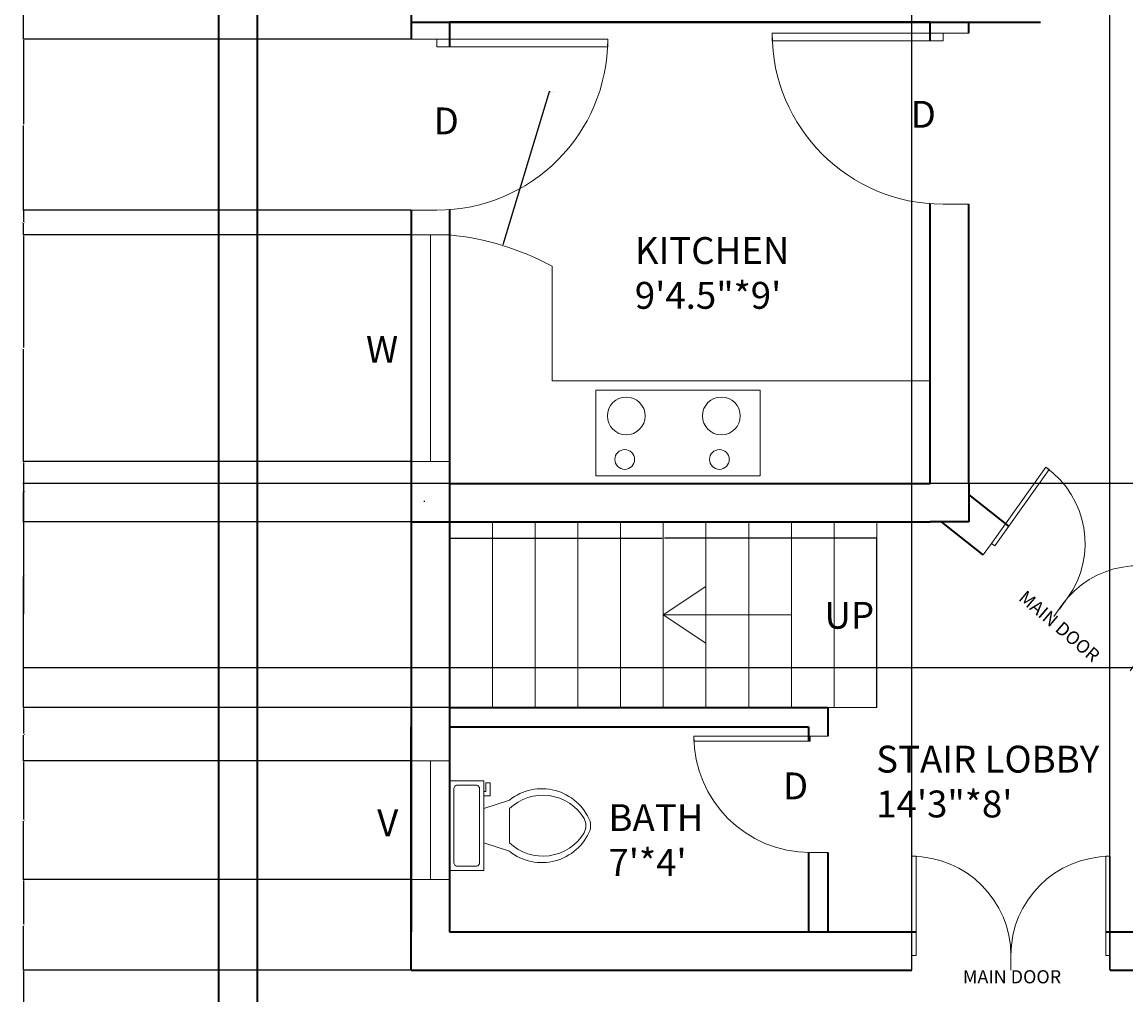
# Model space of a CAD drawing. Units: inches. Extents: x 2284 to 2815, y 1123 to 1948.
# Tile 2 of 6: x 2284 to 2543, y 1414 to 1641. Entities that reach past the tile are written whole.
import ezdxf

# ---------------------------------------------------------------- set-up
doc = ezdxf.new("R2010")
doc.units = ezdxf.units.IN
for name, color, linetype, lineweight in [('A-ANNO-DIMS', 2, 'Continuous', 18), ('A-ANNO-SYMB', 30, 'Continuous', 18), ('A-AREA-IDEN', 30, 'Continuous', 18), ('A-EQPM', 10, 'Continuous', 18), ('A-FLOR-CASE', 8, 'Continuous', 18), ('A-FLOR-FIXT', 9, 'Continuous', 18), ('A-FLOR-STRS', 7, 'Continuous', 18), ('A-WALL-PATT', 140, 'Continuous', 13), ('C-SITE-WALL', 7, 'Continuous', 35), ('DOOR', 190, 'Continuous', 18), ('TEXT', 30, 'Continuous', 18), ('WALL', 7, 'Continuous', 35), ('WIND', 210, 'Continuous', 18)]:
    doc.layers.add(name, color=color, linetype=linetype, lineweight=lineweight)
doc.styles.get("Standard").update_dxf_attribs({"font": 'arial.ttf'})
doc.dimstyles.get("Standard").update_dxf_attribs({"dimtxt": 0.18, "dimasz": 0.18, "dimexe": 0.18, "dimexo": 0.0625, "dimgap": 0.09, "dimtad": 0, "dimtih": 1, "dimtoh": 1, "dimdec": 4, "dimzin": 0, "dimdsep": 46, "dimtxsty": 'Standard', "dimcen": 0.09, "dimadec": 0, "dimazin": 0, "dimtfac": 1, "dimtdec": 4, "dimtofl": 0, "dimtmove": 0, "dimatfit": 3, "dimfxl": 1, "dimtolj": 1, "dimtzin": 0, "dimarcsym": 0})

# ---------------------------------------------------------------- blocks, each defined once
blk = doc.blocks.new('*U2')
for p, q in [((0, 0), (0, -6)), ((40, 0), (40, -6))]:
    blk.add_line(p, q)
blk.add_lwpolyline([(0, 0), (0, 40), (1.75, 40), (1.75, 0)], close=True)
blk.add_arc((0, 0), 40, 0, 90)
blk = doc.blocks.new('*U4')
for p, q in [((9.5, -6), (9.5, -2)), ((-10, -8.5), (-8, -8.5)), ((-10, -9.5), (-10, -8.5)), ((-7, -9.5), (-10, -9.5)), ((-8, -8.5), (-8, -8)), ((-7, -8), (-7, -9.5)), ((-4, -8), (-6, -14)), ((4, -8), (6, -14)), ((4, -14), (-4, -14))]:
    blk.add_line(p, q)
blk.add_lwpolyline([(10.5, -8), (10.5, 0), (-10.5, 0), (-10.5, -8)], close=True)
for points in [[(-9.5, -2), (-9.5, -6)], [(8.5, -1), (-8.5, -1)], [(-8.5, -7), (8.5, -7)]]:
    blk.add_lwpolyline(points)
for centre, radius, start, end in [((-8.62, -1.88), 0.884, 81.8699, 188.1301), ((8.62, -1.88), 0.884, 351.8699, 98.1301), ((-8.62, -6.12), 0.884, 171.8699, 278.1301), ((8.62, -6.12), 0.884, 261.8699, 8.1301), ((3.52, -21.58), 12.17, 141.4691, 247.9714), ((4.2, -21.82), 11.33, 136.3677, 238.9468), ((-3.52, -21.58), 12.17, 292.0284, 38.5307), ((-4.2, -21.82), 11.33, 301.053, 43.6321), ((0, -27.88), 4, 245.7318, 294.2682), ((0, -29), 4, 254.8605, 285.1395)]:
    blk.add_arc(centre, radius, start, end)
blk = doc.blocks.new('*D23')
at = {"layer": 'A-ANNO-DIMS', "color": 0, "lineweight": -2, "transparency": 16777216}
for p, q in [((2375.49, 1419.4), (2284.67, 1419.4)), ((2284.85, 1419.22), (2284.85, 1334.09)), ((2284.85, 1248.6), (2284.85, 1333.73)), ((2339.49, 1248.42), (2284.67, 1248.42))]:
    blk.add_line(p, q, dxfattribs=at)
at = {"layer": 'A-ANNO-DIMS', "color": 0, "transparency": 16777216}
for points in [[(2284.82, 1419.22), (2284.88, 1419.22), (2284.85, 1419.4)], [(2284.82, 1248.6), (2284.88, 1248.6), (2284.85, 1248.42)]]:
    blk.add_solid(points, dxfattribs=at)
at = {"layer": 'Defpoints', "color": 0, "transparency": 16777216}
for p in [(2284.85, 1419.4), (2375.55, 1419.4), (2339.55, 1248.42)]:
    blk.add_point(p, dxfattribs=at)
at = {"layer": 'A-ANNO-DIMS', "color": 0, "transparency": 16777216, "insert": (2284.85, 1333.91), "char_height": 0.18, "attachment_point": 5}
blk.add_mtext('\\A1;171', dxfattribs=at)
blk = doc.blocks.new('*D24')
at = {"layer": 'A-ANNO-DIMS', "color": 0, "lineweight": -2, "transparency": 16777216}
for p, q in [((2375.49, 1440.64), (2284.67, 1440.64)), ((2284.85, 1440.46), (2284.85, 1430.2)), ((2284.85, 1419.58), (2284.85, 1429.84)), ((2375.49, 1419.4), (2284.67, 1419.4))]:
    blk.add_line(p, q, dxfattribs=at)
at = {"layer": 'A-ANNO-DIMS', "color": 0, "transparency": 16777216}
for points in [[(2284.82, 1440.46), (2284.88, 1440.46), (2284.85, 1440.64)], [(2284.82, 1419.58), (2284.88, 1419.58), (2284.85, 1419.4)]]:
    blk.add_solid(points, dxfattribs=at)
at = {"layer": 'Defpoints', "color": 0, "transparency": 16777216}
for p in [(2284.85, 1440.64), (2375.55, 1440.64), (2375.55, 1419.4)]:
    blk.add_point(p, dxfattribs=at)
at = {"layer": 'A-ANNO-DIMS', "color": 0, "transparency": 16777216, "insert": (2284.85, 1430.02), "char_height": 0.18, "attachment_point": 5}
blk.add_mtext('\\A1;21.24', dxfattribs=at)
blk = doc.blocks.new('*D25')
at = {"layer": 'A-ANNO-DIMS', "color": 0, "lineweight": -2, "transparency": 16777216}
for p, q in [((2375.49, 1468.42), (2284.67, 1468.42)), ((2284.85, 1468.24), (2284.85, 1454.71)), ((2284.85, 1440.82), (2284.85, 1454.35)), ((2375.49, 1440.64), (2284.67, 1440.64))]:
    blk.add_line(p, q, dxfattribs=at)
at = {"layer": 'A-ANNO-DIMS', "color": 0, "transparency": 16777216}
for points in [[(2284.82, 1468.24), (2284.88, 1468.24), (2284.85, 1468.42)], [(2284.82, 1440.82), (2284.88, 1440.82), (2284.85, 1440.64)]]:
    blk.add_solid(points, dxfattribs=at)
at = {"layer": 'Defpoints', "color": 0, "transparency": 16777216}
for p in [(2284.85, 1468.42), (2375.55, 1468.42), (2375.55, 1440.64)]:
    blk.add_point(p, dxfattribs=at)
at = {"layer": 'A-ANNO-DIMS', "color": 0, "transparency": 16777216, "insert": (2284.85, 1454.53), "char_height": 0.18, "attachment_point": 5}
blk.add_mtext('\\A1;27.78', dxfattribs=at)
blk = doc.blocks.new('*D26')
at = {"layer": 'A-ANNO-DIMS', "color": 0, "lineweight": -2, "transparency": 16777216}
for p, q in [((2384.49, 1480.9), (2284.67, 1480.9)), ((2284.85, 1480.72), (2284.85, 1474.85)), ((2284.85, 1468.6), (2284.85, 1474.48)), ((2375.49, 1468.42), (2284.67, 1468.42))]:
    blk.add_line(p, q, dxfattribs=at)
at = {"layer": 'A-ANNO-DIMS', "color": 0, "transparency": 16777216}
for points in [[(2284.82, 1480.72), (2284.88, 1480.72), (2284.85, 1480.9)], [(2284.82, 1468.6), (2284.88, 1468.6), (2284.85, 1468.42)]]:
    blk.add_solid(points, dxfattribs=at)
at = {"layer": 'Defpoints', "color": 0, "transparency": 16777216}
for p in [(2284.85, 1480.9), (2384.55, 1480.9), (2375.55, 1468.42)]:
    blk.add_point(p, dxfattribs=at)
at = {"layer": 'A-ANNO-DIMS', "color": 0, "transparency": 16777216, "insert": (2284.85, 1474.66), "char_height": 0.18, "attachment_point": 5}
blk.add_mtext('\\A1;12.48', dxfattribs=at)
blk = doc.blocks.new('*D27')
at = {"layer": 'A-ANNO-DIMS', "color": 0, "lineweight": -2, "transparency": 16777216}
for p, q in [((2384.49, 1524.4), (2284.67, 1524.4)), ((2284.85, 1524.22), (2284.85, 1502.84)), ((2284.85, 1481.08), (2284.85, 1502.47)), ((2384.49, 1480.9), (2284.67, 1480.9))]:
    blk.add_line(p, q, dxfattribs=at)
at = {"layer": 'A-ANNO-DIMS', "color": 0, "transparency": 16777216}
for points in [[(2284.82, 1524.22), (2284.88, 1524.22), (2284.85, 1524.4)], [(2284.82, 1481.08), (2284.88, 1481.08), (2284.85, 1480.9)]]:
    blk.add_solid(points, dxfattribs=at)
at = {"layer": 'Defpoints', "color": 0, "transparency": 16777216}
for p in [(2284.85, 1524.4), (2384.55, 1524.4), (2384.55, 1480.9)]:
    blk.add_point(p, dxfattribs=at)
at = {"layer": 'A-ANNO-DIMS', "color": 0, "transparency": 16777216, "insert": (2284.85, 1502.65), "char_height": 0.18, "attachment_point": 5}
blk.add_mtext('\\A1;43.5', dxfattribs=at)
blk = doc.blocks.new('*D28')
at = {"layer": 'A-ANNO-DIMS', "color": 0, "lineweight": -2, "transparency": 16777216}
for p, q in [((2375.49, 1538.49), (2284.67, 1538.49)), ((2284.85, 1538.31), (2284.85, 1531.63)), ((2284.85, 1524.58), (2284.85, 1531.26)), ((2384.49, 1524.4), (2284.67, 1524.4))]:
    blk.add_line(p, q, dxfattribs=at)
at = {"layer": 'A-ANNO-DIMS', "color": 0, "transparency": 16777216}
for points in [[(2284.82, 1538.31), (2284.88, 1538.31), (2284.85, 1538.49)], [(2284.82, 1524.58), (2284.88, 1524.58), (2284.85, 1524.4)]]:
    blk.add_solid(points, dxfattribs=at)
at = {"layer": 'Defpoints', "color": 0, "transparency": 16777216}
for p in [(2284.85, 1538.49), (2375.55, 1538.49), (2384.55, 1524.4)]:
    blk.add_point(p, dxfattribs=at)
at = {"layer": 'A-ANNO-DIMS', "color": 0, "transparency": 16777216, "insert": (2284.85, 1531.45), "char_height": 0.18, "attachment_point": 5}
blk.add_mtext('\\A1;14.086', dxfattribs=at)
blk = doc.blocks.new('*D29')
at = {"layer": 'A-ANNO-DIMS', "color": 0, "lineweight": -2, "transparency": 16777216}
for p, q in [((2375.49, 1591.56), (2284.67, 1591.56)), ((2284.85, 1591.38), (2284.85, 1565.21)), ((2284.85, 1538.67), (2284.85, 1564.84)), ((2375.49, 1538.49), (2284.67, 1538.49))]:
    blk.add_line(p, q, dxfattribs=at)
at = {"layer": 'A-ANNO-DIMS', "color": 0, "transparency": 16777216}
for points in [[(2284.82, 1591.38), (2284.88, 1591.38), (2284.85, 1591.56)], [(2284.82, 1538.67), (2284.88, 1538.67), (2284.85, 1538.49)]]:
    blk.add_solid(points, dxfattribs=at)
at = {"layer": 'Defpoints', "color": 0, "transparency": 16777216}
for p in [(2284.85, 1591.56), (2375.55, 1591.56), (2375.55, 1538.49)]:
    blk.add_point(p, dxfattribs=at)
at = {"layer": 'A-ANNO-DIMS', "color": 0, "transparency": 16777216, "insert": (2284.85, 1565.03), "char_height": 0.18, "attachment_point": 5}
blk.add_mtext('\\A1;53.07', dxfattribs=at)
blk = doc.blocks.new('*D30')
at = {"layer": 'A-ANNO-DIMS', "color": 0, "lineweight": -2, "transparency": 16777216}
for p, q in [((2375.49, 1597.37), (2284.67, 1597.37)), ((2284.85, 1597.19), (2284.85, 1594.65)), ((2284.85, 1591.74), (2284.85, 1594.29)), ((2375.49, 1591.56), (2284.67, 1591.56))]:
    blk.add_line(p, q, dxfattribs=at)
at = {"layer": 'A-ANNO-DIMS', "color": 0, "transparency": 16777216}
for points in [[(2284.82, 1597.19), (2284.88, 1597.19), (2284.85, 1597.37)], [(2284.82, 1591.74), (2284.88, 1591.74), (2284.85, 1591.56)]]:
    blk.add_solid(points, dxfattribs=at)
at = {"layer": 'Defpoints', "color": 0, "transparency": 16777216}
for p in [(2284.85, 1597.37), (2375.55, 1597.37), (2375.55, 1591.56)]:
    blk.add_point(p, dxfattribs=at)
at = {"layer": 'A-ANNO-DIMS', "color": 0, "transparency": 16777216, "insert": (2284.85, 1594.47), "char_height": 0.18, "attachment_point": 5}
blk.add_mtext('\\A1;5.807', dxfattribs=at)
blk = doc.blocks.new('*D31')
at = {"layer": 'A-ANNO-DIMS', "color": 0, "lineweight": -2, "transparency": 16777216}
for p, q in [((2375.49, 1637.37), (2284.67, 1637.37)), ((2284.85, 1637.19), (2284.85, 1617.55)), ((2284.85, 1597.55), (2284.85, 1617.19)), ((2375.49, 1597.37), (2284.67, 1597.37))]:
    blk.add_line(p, q, dxfattribs=at)
at = {"layer": 'A-ANNO-DIMS', "color": 0, "transparency": 16777216}
for points in [[(2284.82, 1637.19), (2284.88, 1637.19), (2284.85, 1637.37)], [(2284.82, 1597.55), (2284.88, 1597.55), (2284.85, 1597.37)]]:
    blk.add_solid(points, dxfattribs=at)
at = {"layer": 'Defpoints', "color": 0, "transparency": 16777216}
for p in [(2284.85, 1637.37), (2375.55, 1637.37), (2375.55, 1597.37)]:
    blk.add_point(p, dxfattribs=at)
at = {"layer": 'A-ANNO-DIMS', "color": 0, "transparency": 16777216, "insert": (2284.85, 1617.37), "char_height": 0.18, "attachment_point": 5}
blk.add_mtext('\\A1;40', dxfattribs=at)
blk = doc.blocks.new('*D32')
at = {"layer": 'A-ANNO-DIMS', "color": 0, "lineweight": -2, "transparency": 16777216}
for p, q in [((2375.49, 1678.06), (2284.67, 1678.06)), ((2284.85, 1677.88), (2284.85, 1657.9)), ((2284.85, 1637.55), (2284.85, 1657.53)), ((2375.49, 1637.37), (2284.67, 1637.37))]:
    blk.add_line(p, q, dxfattribs=at)
at = {"layer": 'A-ANNO-DIMS', "color": 0, "transparency": 16777216}
for points in [[(2284.82, 1677.88), (2284.88, 1677.88), (2284.85, 1678.06)], [(2284.82, 1637.55), (2284.88, 1637.55), (2284.85, 1637.37)]]:
    blk.add_solid(points, dxfattribs=at)
at = {"layer": 'Defpoints', "color": 0, "transparency": 16777216}
for p in [(2284.85, 1678.06), (2375.55, 1678.06), (2375.55, 1637.37)]:
    blk.add_point(p, dxfattribs=at)
at = {"layer": 'A-ANNO-DIMS', "color": 0, "transparency": 16777216, "insert": (2284.85, 1657.71), "char_height": 0.18, "attachment_point": 5}
blk.add_mtext('\\A1;40.69', dxfattribs=at)
blk = doc.blocks.new('*D46')
at = {"layer": 'A-ANNO-DIMS', "color": 0, "lineweight": -2, "transparency": 16777216}
for p, q in [((2492.72, 1419.47), (2492.72, 1948.28)), ((2539.13, 1419.47), (2539.13, 1948.28)), ((2492.9, 1948.1), (2515.54, 1948.1)), ((2538.95, 1948.1), (2516.3, 1948.1))]:
    blk.add_line(p, q, dxfattribs=at)
at = {"layer": 'A-ANNO-DIMS', "color": 0, "transparency": 16777216}
for points in [[(2492.9, 1948.13), (2492.9, 1948.07), (2492.72, 1948.1)], [(2538.95, 1948.13), (2538.95, 1948.07), (2539.13, 1948.1)]]:
    blk.add_solid(points, dxfattribs=at)
at = {"layer": 'Defpoints', "color": 0, "transparency": 16777216}
for p in [(2539.13, 1948.1), (2492.72, 1419.4), (2539.13, 1419.4)]:
    blk.add_point(p, dxfattribs=at)
at = {"layer": 'A-ANNO-DIMS', "color": 0, "transparency": 16777216, "insert": (2515.92, 1948.1), "char_height": 0.18, "attachment_point": 5}
blk.add_mtext('\\A1;46.41', dxfattribs=at)
blk = doc.blocks.new('*D55')
at = {"layer": 'A-ANNO-DIMS', "color": 0, "lineweight": -2, "transparency": 16777216}
for p, q in [((2599.47, 1533.4), (2284.67, 1533.4)), ((2284.85, 1533.22), (2284.85, 1511.99)), ((2284.85, 1490.38), (2284.85, 1511.62)), ((2555.49, 1490.2), (2284.67, 1490.2))]:
    blk.add_line(p, q, dxfattribs=at)
at = {"layer": 'A-ANNO-DIMS', "color": 0, "transparency": 16777216}
for points in [[(2284.82, 1533.22), (2284.88, 1533.22), (2284.85, 1533.4)], [(2284.82, 1490.38), (2284.88, 1490.38), (2284.85, 1490.2)]]:
    blk.add_solid(points, dxfattribs=at)
at = {"layer": 'Defpoints', "color": 0, "transparency": 16777216}
for p in [(2284.85, 1533.4), (2599.53, 1533.4), (2555.55, 1490.2)]:
    blk.add_point(p, dxfattribs=at)
at = {"layer": 'A-ANNO-DIMS', "color": 0, "transparency": 16777216, "insert": (2284.85, 1511.8), "char_height": 0.18, "attachment_point": 5}
blk.add_mtext('\\A1;43.2', dxfattribs=at)
blk = doc.blocks.new('*D56')
at = {"layer": 'A-ANNO-DIMS', "color": 0, "lineweight": -2, "transparency": 16777216}
for p, q in [((2384.55, 1480.97), (2384.55, 1520.78)), ((2384.73, 1520.6), (2434.27, 1520.6)), ((2484.37, 1520.6), (2434.83, 1520.6)), ((2484.55, 1480.97), (2484.55, 1520.78))]:
    blk.add_line(p, q, dxfattribs=at)
at = {"layer": 'A-ANNO-DIMS', "color": 0, "transparency": 16777216}
for points in [[(2384.73, 1520.63), (2384.73, 1520.57), (2384.55, 1520.6)], [(2484.37, 1520.63), (2484.37, 1520.57), (2484.55, 1520.6)]]:
    blk.add_solid(points, dxfattribs=at)
at = {"layer": 'Defpoints', "color": 0, "transparency": 16777216}
for p in [(2484.55, 1520.6), (2384.55, 1480.9), (2484.55, 1480.9)]:
    blk.add_point(p, dxfattribs=at)
at = {"layer": 'A-ANNO-DIMS', "color": 0, "transparency": 16777216, "insert": (2434.55, 1520.6), "char_height": 0.18, "attachment_point": 5}
blk.add_mtext('\\A1;100', dxfattribs=at)
blk = doc.blocks.new('*D60')
at = {"layer": 'A-ANNO-DIMS', "color": 0, "lineweight": -2, "transparency": 16777216}
for p, q in [((2407.89, 1625.05), (2396.98, 1589.29)), ((2408.07, 1625.05), (2407.89, 1625.05)), ((2378.55, 1529.23), (2378.73, 1529.23)), ((2378.64, 1529.14), (2378.64, 1529.32))]:
    blk.add_line(p, q, dxfattribs=at)
at = {"layer": 'A-ANNO-DIMS', "color": 0, "transparency": 16777216}
blk.add_solid([(2396.95, 1589.3), (2397.01, 1589.28), (2396.93, 1589.12)], dxfattribs=at)
at = {"layer": 'Defpoints', "color": 0, "transparency": 16777216}
for p in [(2396.93, 1589.12), (2378.64, 1529.23)]:
    blk.add_point(p, dxfattribs=at)
at = {"layer": 'A-ANNO-DIMS', "color": 0, "transparency": 16777216, "insert": (2408.54, 1625.05), "char_height": 0.18, "attachment_point": 5}
blk.add_mtext('\\A1;R62.61', dxfattribs=at)

msp = doc.modelspace()

# ---------------------------------------------------------------- hatches: boundary and pattern name
at = {"layer": 'A-WALL-PATT'}
h = msp.add_hatch(dxfattribs=at)
h.set_pattern_fill('AR-SAND', color=256, scale=8.5)
h.paths.add_polyline_path([(2339.554, 1899.404), (2375.554, 1899.404), (2765.554, 1899.404), (2765.554, 1185.404), (2549.3222, 1185.404), (2549.3222, 1176.404), (2774.554, 1176.404), (2774.554, 1908.404), (2330.554, 1908.404), (2330.554, 1176.404), (2349.4276, 1176.404), (2349.4276, 1185.404), (2339.554, 1185.404)])
h.paths.add_polyline_path([(2710.054, 1899.404), (2701.054, 1899.404), (2701.054, 1889.8374), (2710.054, 1889.8374)], flags=17)
h = msp.add_hatch(dxfattribs=at)
h.set_pattern_fill('AR-SAND', color=256, scale=8.5)
h.paths.add_polyline_path([(2549.554, 1863.404), (2375.554, 1863.404), (2375.554, 1840.6021), (2384.554, 1840.6021), (2384.554, 1854.404), (2480.554, 1854.404), (2549.554, 1854.404)])
h.paths.add_polyline_path([(2384.554, 1795.904), (2384.554, 1809.1528), (2375.554, 1809.1528), (2375.554, 1758.7416), (2384.554, 1758.7416)])
h.paths.add_polyline_path([(2549.554, 1836.404), (2549.554, 1854.404), (2540.554, 1854.404), (2540.554, 1800.404), (2485.054, 1800.404), (2485.054, 1802.7347), (2480.554, 1802.7347), (2480.554, 1800.404), (2384.554, 1800.404), (2384.554, 1795.904), (2485.054, 1795.904), (2540.554, 1795.904), (2540.554, 1678.5102), (2543.2164, 1676.3784), (2547.9, 1672.6283), (2549.554, 1677.404), (2549.554, 1795.904)])
h.paths.add_polyline_path([(2452.31, 1803.9815), (2480.7795, 1803.9815), (2480.7795, 1802.7347), (2452.2828, 1802.7347), (2452.2828, 1803.9815), (2452.31, 1803.9815, -0.39915744), (2480.554, 1831.2306), (2480.554, 1854.404), (2540.554, 1854.404), (2485.054, 1837.4988), (2485.054, 1831.2315), (2480.7795, 1831.2315, 0.40145271)], flags=17)
h.paths.add_polyline_path([(2583.189, 1845.404), (2549.554, 1845.404), (2549.554, 1836.404), (2583.189, 1836.404)])
h.paths.add_polyline_path([(2710.054, 1858.3882), (2701.054, 1858.3882), (2701.054, 1845.404), (2671.4007, 1845.404), (2671.4007, 1836.404), (2710.054, 1836.404)])
h.paths.add_polyline_path([(2710.054, 1836.404), (2705.554, 1836.404), (2705.554, 1774.904), (2710.054, 1774.904), (2710.054, 1779.404)])
h.paths.add_polyline_path([(2765.554, 1779.404), (2737.9116, 1779.404, -0.00645116), (2737.9201, 1778.7436), (2737.9201, 1774.904), (2765.554, 1774.904)])
h.paths.add_polyline_path([(2712.3231, 1778.7436), (2712.3231, 1779.404), (2710.054, 1779.404), (2710.054, 1774.904), (2712.3231, 1774.904)])
h.paths.add_polyline_path([(2710.054, 1774.904), (2705.554, 1774.904), (2705.554, 1769.4647), (2710.054, 1769.4647)])
h.paths.add_polyline_path([(2710.054, 1702.7233), (2705.554, 1702.7233), (2705.554, 1686.404), (2592.0733, 1686.404, -0.01876983), (2592.186, 1683.404), (2592.186, 1677.404), (2705.554, 1677.404), (2765.554, 1677.404), (2765.554, 1686.404), (2710.054, 1686.404)])
h.paths.add_polyline_path([(2384.554, 1641.404), (2375.554, 1641.404), (2375.554, 1637.3708), (2381.554, 1637.3708), (2384.554, 1637.3708)])
h.paths.add_polyline_path([(2384.554, 1678.0573), (2375.554, 1678.0573), (2375.554, 1641.404), (2384.554, 1641.404), (2522.8991, 1641.404), (2518.2155, 1645.1541, -0.00736412), (2517.3067, 1645.904), (2384.554, 1645.904)])
h.paths.add_polyline_path([(2384.554, 1597.4834, -0.01876983), (2381.554, 1597.3708), (2375.554, 1597.3708), (2375.554, 1591.564), (2384.554, 1591.564)])
h.paths.add_polyline_path([(2384.554, 1533.404), (2384.554, 1538.4896), (2375.554, 1538.4896), (2375.554, 1524.404), (2384.554, 1524.404)])
h.paths.add_polyline_path([(2506.054, 1533.404), (2506.054, 1598.7748), (2500.054, 1598.7748, -0.01876983), (2497.054, 1598.8874), (2497.054, 1533.404), (2384.554, 1533.404), (2384.554, 1524.404), (2497.054, 1524.404), (2506.054, 1524.404)])
h.paths.add_polyline_path([(2473.054, 1446.985), (2468.9674, 1446.985, -0.00379375), (2468.554, 1446.9881), (2468.554, 1428.404), (2473.054, 1428.404)])
h.paths.add_polyline_path([(2384.554, 1524.404), (2375.554, 1524.404), (2375.554, 1468.4232), (2384.554, 1468.4232)])
h.paths.add_polyline_path([(2473.054, 1480.904), (2384.554, 1480.904), (2384.554, 1476.404), (2468.554, 1476.404), (2468.554, 1474.2289), (2468.9674, 1474.2289), (2473.054, 1474.2289)])
h.paths.add_polyline_path([(2555.554, 1428.404), (2546.554, 1428.404), (2539.1317, 1428.404), (2539.1317, 1422.885), (2539.1317, 1419.404), (2546.554, 1419.404), (2555.554, 1419.404)])
h.paths.add_polyline_path([(2564.554, 1368.404), (2564.554, 1370.9838), (2561.554, 1370.9838), (2555.554, 1370.9838), (2555.554, 1359.404), (2564.554, 1359.404)])
h.paths.add_polyline_path([(2623.1768, 1368.404), (2564.554, 1368.404), (2564.554, 1359.404), (2623.1768, 1359.404)])
h.paths.add_polyline_path([(2492.7181, 1422.885), (2492.7181, 1428.404), (2384.554, 1428.404), (2384.554, 1440.6426), (2375.554, 1440.6426), (2375.554, 1419.404), (2492.7181, 1419.404)])
h.paths.add_polyline_path([(2765.554, 1368.404), (2710.406, 1368.404), (2710.406, 1359.404), (2765.554, 1359.404)])
h.paths.add_polyline_path([(2765.554, 1533.404), (2732.876, 1533.404), (2732.876, 1524.404), (2765.554, 1524.404)])
h.paths.add_polyline_path([(2624.1792, 1533.404), (2599.5288, 1533.404), (2590.3672, 1524.404), (2564.554, 1499.046), (2555.554, 1490.2048), (2555.554, 1410.9838), (2561.554, 1410.9838, -0.01876983), (2564.554, 1410.8712), (2564.554, 1486.4298), (2603.2099, 1524.404), (2624.1792, 1524.404)])
h.paths.add_polyline_path([(2555.554, 1490.2048), (2556.4043, 1491.0401), (2549.047, 1496.8538), (2545.7227, 1492.1958), (2543.8126, 1489.5193), (2555.554, 1480.2413)])
h.paths.add_polyline_path([(2514.6892, 1524.0031), (2506.054, 1530.8266), (2506.054, 1524.404), (2499.6656, 1524.404), (2500.474, 1523.7652), (2509.4548, 1516.6686), (2511.3649, 1519.3451)])
h.paths.add_polyline_path([(2365.9834, 1447.3726), (2374.9891, 1447.3726), (2374.9891, 1460.3342), (2365.9834, 1460.3342)], flags=9)
h.paths.add_polyline_path([(2366.9945, 1818.7713), (2376.0002, 1818.7713), (2376.0002, 1831.7328), (2366.9945, 1831.7328)], flags=9)
h.paths.add_polyline_path([(2363.2989, 1558.2059), (2374.7373, 1558.2059), (2374.7373, 1571.1674), (2363.2989, 1571.1674)], flags=9)
h.paths.add_polyline_path([(2364.8137, 1707.1012), (2376.2521, 1707.1012), (2376.2521, 1720.0627), (2364.8137, 1720.0627)], flags=9)
h.paths.add_polyline_path([(2460.3189, 1455.9932), (2469.8094, 1455.9932), (2469.8094, 1468.9547), (2460.3189, 1468.9547)], flags=9)
h.paths.add_polyline_path([(2558.6325, 1386.2225), (2568.1231, 1386.2225), (2568.1231, 1399.184), (2558.6325, 1399.184)], flags=9)
h.paths.add_polyline_path([(2378.5629, 1611.6816), (2388.0534, 1611.6816), (2388.0534, 1624.6431), (2378.5629, 1624.6431)], flags=9)
h.paths.add_polyline_path([(2490.2277, 1613.2326), (2499.7182, 1613.2326), (2499.7182, 1626.1941), (2490.2277, 1626.1941)], flags=9)
h.paths.add_polyline_path([(2522.9652, 1656.7942), (2532.4557, 1656.7942), (2532.4557, 1669.7557), (2522.9652, 1669.7557)], flags=9)
h.paths.add_polyline_path([(2567.5462, 1677.3031), (2577.0367, 1677.3031), (2577.0367, 1690.2646), (2567.5462, 1690.2646)], flags=9)
h.paths.add_polyline_path([(2363.196, 1676.9136), (2363.196, 1756.4461), (2350.2345, 1756.4461), (2350.2345, 1676.9136)], flags=9)
h.paths.add_polyline_path([(2515.5569, 1505.5998), (2535.7182, 1488.4964), (2539.8301, 1493.3434), (2519.6687, 1510.4468)], flags=9)
h.paths.add_polyline_path([(2503.6006, 1414.6146), (2530.0393, 1414.6146), (2530.0393, 1420.9707), (2503.6006, 1420.9707)], flags=9)
h.paths.add_polyline_path([(2391.2946, 1877.326), (2470.827, 1877.326), (2470.827, 1890.2876), (2391.2946, 1890.2876)], flags=9)
h.paths.add_polyline_path([(2580.3233, 1794.4386), (2629.1831, 1794.4386), (2629.1831, 1817.9089), (2580.3233, 1817.9089)], flags=9)
h.paths.add_polyline_path([(2585.6043, 1595.2228), (2648.3653, 1595.2228), (2648.3653, 1618.6931), (2585.6043, 1618.6931)], flags=9)
h.paths.add_polyline_path([(2591.9981, 1445.0189), (2637.889, 1445.0189), (2637.889, 1468.4892), (2591.9981, 1468.4892)], flags=9)
h.paths.add_polyline_path([(2459.0727, 1376.5795), (2515.4624, 1376.5795), (2515.4624, 1400.0498), (2459.0727, 1400.0498)], flags=9)
h.paths.add_polyline_path([(2481.8769, 1451.6363), (2543.2049, 1451.6363), (2543.2049, 1475.1066), (2481.8769, 1475.1066)], flags=9)
h.paths.add_polyline_path([(2470.0329, 1495.943), (2485.3842, 1495.943), (2485.3842, 1508.9045), (2470.0329, 1508.9045)], flags=9)
h.paths.add_polyline_path([(2419.5143, 1438.0898), (2446.0938, 1438.0898), (2446.0938, 1461.5344), (2419.5143, 1461.5344)], flags=9)
h.paths.add_polyline_path([(2425.6893, 1570.7133), (2467.4012, 1570.7133), (2467.4012, 1594.1836), (2425.6893, 1594.1836)], flags=25)
h.paths.add_polyline_path([(2428.101, 1758.2973), (2476.9609, 1758.2973), (2476.9609, 1781.7676), (2428.101, 1781.7676)], flags=25)

# ---------------------------------------------------------------- linework, layer by layer
at = {"layer": 'A-ANNO-SYMB'}
for p, q in [((2434.554, 1502.654), (2444.554, 1509.2875)), ((2464.554, 1502.654), (2434.554, 1502.654)), ((2434.554, 1502.654), (2444.554, 1496.0204))]:
    msp.add_line(p, q, dxfattribs=at)
at = {"layer": 'A-EQPM'}
msp.add_lwpolyline([(2418.7835, 1555.2071), (2457.2539, 1555.2071), (2457.2539, 1535.1902), (2418.7835, 1535.1902)], close=True, dxfattribs=at)
for centre, radius in [((2425.9122, 1549.1898), 4.4209), ((2448.1587, 1549.1898), 4.4209), ((2425.5435, 1538.9971), 2.3072), ((2447.6985, 1538.9971), 2.3072)]:
    msp.add_circle(centre, radius, dxfattribs=at)
at = {"layer": 'A-FLOR-CASE'}
for p, q in [((2408.554, 1584.2376), (2408.554, 1557.404)), ((2497.054, 1557.404), (2408.554, 1557.404)), ((2497.054, 1533.404), (2497.054, 1557.404))]:
    msp.add_line(p, q, dxfattribs=at)
msp.add_arc((2378.6445, 1529.2322), 62.6113, 61.464659, 84.584168, dxfattribs=at)
at = {"layer": 'A-FLOR-STRS'}
for p, q in [((2384.554, 1480.904), (2384.554, 1524.404)), ((2394.554, 1480.904), (2394.554, 1524.404)), ((2404.554, 1480.904), (2404.554, 1524.404)), ((2414.554, 1480.904), (2414.554, 1524.404)), ((2424.554, 1480.904), (2424.554, 1524.404)), ((2434.554, 1480.904), (2434.554, 1524.404)), ((2444.554, 1480.904), (2444.554, 1524.404)), ((2454.554, 1480.904), (2454.554, 1524.404)), ((2464.554, 1480.904), (2464.554, 1524.404)), ((2474.554, 1480.904), (2474.554, 1524.404)), ((2484.554, 1480.904), (2484.554, 1524.404)), ((2473.054, 1480.904), (2484.554, 1480.904))]:
    msp.add_line(p, q, dxfattribs=at)
at = {"layer": 'C-SITE-WALL'}
for p, q in [((2330.554, 1176.404), (2330.554, 1908.404)), ((2339.554, 1185.404), (2339.554, 1899.404))]:
    msp.add_line(p, q, dxfattribs=at)
at = {"layer": 'WALL'}
for p, q in [((2375.554, 1714.7105), (2375.554, 1641.404)), ((2375.554, 1641.404), (2522.8991, 1641.404)), ((2375.554, 1641.404), (2375.554, 1637.3708)), ((2497.054, 1641.404), (2384.554, 1641.404)), ((2384.554, 1641.404), (2384.554, 1635.6208)), ((2497.054, 1637.0248), (2497.054, 1641.404)), ((2506.054, 1638.7748), (2506.054, 1641.404)), ((2375.554, 1597.3708), (2375.554, 1524.404)), ((2384.554, 1597.4834), (2384.554, 1533.404)), ((2497.054, 1533.404), (2497.054, 1598.8874)), ((2506.054, 1533.404), (2506.054, 1598.7748)), ((2384.554, 1533.404), (2497.054, 1533.404)), ((2384.554, 1533.404), (2384.554, 1524.404)), ((2506.054, 1533.404), (2506.054, 1524.404)), ((2515.4426, 1523.4078), (2506.054, 1530.8266)), ((2375.554, 1524.404), (2497.054, 1524.404)), ((2375.554, 1524.404), (2375.554, 1428.404)), ((2384.554, 1524.404), (2384.554, 1428.404)), ((2506.054, 1524.404), (2497.054, 1524.404)), ((2500.474, 1523.7652), (2499.6656, 1524.404)), ((2509.4548, 1516.6686), (2500.474, 1523.7652)), ((2384.554, 1480.904), (2473.054, 1480.904)), ((2473.054, 1480.904), (2473.054, 1474.2289)), ((2375.554, 1419.404), (2375.554, 1476.404)), ((2384.554, 1476.404), (2468.554, 1476.404)), ((2468.554, 1476.404), (2468.554, 1473.037)), ((2468.554, 1446.9881), (2468.554, 1428.404)), ((2473.054, 1446.985), (2473.054, 1428.404)), ((2384.554, 1428.404), (2493.7334, 1428.404)), ((2538.1164, 1428.404), (2546.554, 1428.404)), ((2375.554, 1419.404), (2492.7181, 1419.404)), ((2539.1317, 1419.404), (2546.554, 1419.404))]:
    msp.add_line(p, q, dxfattribs=at)
at = {"layer": 'WIND'}
for p, q in [((2380.054, 1538.4896), (2380.054, 1591.564)), ((2380.054, 1440.6426), (2380.054, 1468.4232))]:
    msp.add_line(p, q, dxfattribs=at)
for points in [[(2384.554, 1538.4896), (2375.554, 1538.4896), (2375.554, 1591.564), (2384.554, 1591.564)], [(2384.554, 1440.6426), (2375.554, 1440.6426), (2375.554, 1468.4232), (2384.554, 1468.4232)]]:
    msp.add_lwpolyline(points, close=True, dxfattribs=at)

# ---------------------------------------------------------------- block references
at = {"layer": 'A-FLOR-FIXT', "xscale": -1, "rotation": 90}
msp.add_blockref('*U4', (2384.554, 1453.2663), dxfattribs=at)
at = {"layer": 'DOOR', "xscale": -1, "rotation": 90}
msp.add_blockref('*U2', (2500.054, 1638.7748), dxfattribs=at)
at = {"layer": 'DOOR', "rotation": 270}
msp.add_blockref('*U2', (2381.554, 1637.3708), dxfattribs=at)
at = {"layer": 'DOOR'}
for p, xscale, yscale, zscale, rotation in [((2511.3649, 1519.3451), 0.5480269300903049, 0.5480269300903049, 0.5480269300903049, 324.4855940870744), ((2545.7227, 1492.1958), -0.5480269300903049, 0.5480269300903049, 0.5480269300903049, 324.4855940870744), ((2468.9674, 1474.2289), -0.68109853698985, 0.68109853698985, 0.68109853698985, 90)]:
    msp.add_blockref('*U2', p, dxfattribs=dict(at, xscale=xscale, yscale=yscale, zscale=zscale, rotation=rotation))
at = {"layer": 'DOOR', "yscale": 0.5801697227689644, "zscale": 0.5801697227689644}
for p, xscale in [((2492.7181, 1422.885), 0.5801697227689644), ((2539.1317, 1422.885), -0.5801697227689644)]:
    msp.add_blockref('*U2', p, dxfattribs=dict(at, xscale=xscale))

# ---------------------------------------------------------------- texts
at = {"layer": 'A-ANNO-SYMB', "insert": (2472.2961, 1505.6674), "char_height": 6.28983, "attachment_point": 1}
msp.add_mtext_dynamic_manual_height_columns('UP', width=114.078767, gutter_width=31.4491, heights=[0], dxfattribs=at)
at = {"layer": 'A-AREA-IDEN', "attachment_point": 1}
for s, insert, char_height in [('KITCHEN\\P9\'4.5"*9\'', (2427.9053, 1591.0537), 6.28983), ('STAIR LOBBY\\P14\'3"*8\'', (2484.4061, 1471.981), 6.289829), ("BATH\\P7'*4'", (2421.7303, 1458.2972), 6.28983)]:
    msp.add_mtext_dynamic_manual_height_columns(s, width=114.078767, gutter_width=31.4491, heights=[0], dxfattribs=dict(at, insert=insert, char_height=char_height))
at = {"layer": 'TEXT', "attachment_point": 1}
for s, width, gutter_width, insert, char_height in [('D', 114.078767, 31.4491, (2492.4781, 1622.9569), 6.2898), ('D', 114.078767, 31.4491, (2380.8133, 1621.406), 6.2898), ('W', 114.078767, 31.4491, (2364.9786, 1567.9303), 6.2898), ('D', 114.078767, 31.4491, (2462.5693, 1465.7176), 6.2898), ('V', 114.078767, 31.4491, (2367.5944, 1457.097), 6.2898), ('MAIN DOOR', 55.94264, 15.4222, (2504.6915, 1419.438), 3.08444)]:
    msp.add_mtext_dynamic_manual_height_columns(s, width=width, gutter_width=gutter_width, heights=[0], dxfattribs=dict(at, insert=insert, char_height=char_height))
at = {"layer": 'TEXT', "insert": (2519.5091, 1508.5722), "char_height": 3.08444, "attachment_point": 1, "rotation": 319.691145}
msp.add_mtext_dynamic_manual_height_columns('MAIN DOOR', width=55.94264, gutter_width=15.4222, heights=[0], dxfattribs=at)

# ---------------------------------------------------------------- dimensions: what is measured, and where the dimension line sits
at = {"layer": 'A-ANNO-DIMS'}
for base, p1, p2, override, picture, middle in [((2539.1317, 1948.104), (2492.7181, 1419.404), (2539.1317, 1419.404), {"dimdec": 2, "dimlfac": 1, "dimrnd": 0, "dimzin": 0, "dimdsep": 46, "dimlunit": 2}, '*D46', (2515.9249, 1948.104)), ((2484.554, 1520.604), (2384.554, 1480.904), (2484.554, 1480.904), {"dimdec": 0, "dimlfac": 1, "dimrnd": 0, "dimzin": 0, "dimdsep": 46, "dimlunit": 2}, '*D56', (2434.554, 1520.604))]:
    dim = msp.add_linear_dim(base=base, p1=p1, p2=p2, dimstyle='Standard', override=override, dxfattribs=at)
    dim.commit()
    dim.dimension.update_dxf_attribs({"geometry": picture, "text_midpoint": middle})
for base, p1, p2, override, picture, middle in [((2284.854, 1678.0573), (2375.554, 1637.3708), (2375.554, 1678.0573), {"dimdec": 2, "dimlfac": 1, "dimrnd": 0, "dimzin": 0, "dimdsep": 46, "dimlunit": 2}, '*D32', (2284.854, 1657.714)), ((2284.854, 1637.3708), (2375.554, 1597.3708), (2375.554, 1637.3708), {"dimdec": 0, "dimlfac": 1, "dimrnd": 0, "dimzin": 0, "dimdsep": 46, "dimlunit": 2}, '*D31', (2284.854, 1617.3708)), ((2284.854, 1597.3708), (2375.554, 1591.564), (2375.554, 1597.3708), {"dimdec": 3, "dimlfac": 1, "dimrnd": 0, "dimzin": 0, "dimdsep": 46, "dimlunit": 2}, '*D30', (2284.854, 1594.4674)), ((2284.854, 1591.564), (2375.554, 1538.4896), (2375.554, 1591.564), {"dimdec": 2, "dimlfac": 1, "dimrnd": 0, "dimzin": 0, "dimdsep": 46, "dimlunit": 2}, '*D29', (2284.854, 1565.0268)), ((2284.854, 1538.4896), (2384.554, 1524.404), (2375.554, 1538.4896), {"dimdec": 3, "dimlfac": 1, "dimrnd": 0, "dimzin": 0, "dimdsep": 46, "dimlunit": 2}, '*D28', (2284.854, 1531.4468)), ((2284.854, 1533.404), (2555.554, 1490.2048), (2599.5288, 1533.404), {"dimdec": 1, "dimlfac": 1, "dimrnd": 0, "dimzin": 0, "dimdsep": 46, "dimlunit": 2}, '*D55', (2284.854, 1511.8044)), ((2284.854, 1524.404), (2384.554, 1480.904), (2384.554, 1524.404), {"dimdec": 1, "dimlfac": 1, "dimrnd": 0, "dimzin": 0, "dimdsep": 46, "dimlunit": 2}, '*D27', (2284.854, 1502.654)), ((2284.854, 1480.904), (2375.554, 1468.4232), (2384.554, 1480.904), {"dimdec": 2, "dimlfac": 1, "dimrnd": 0, "dimzin": 0, "dimdsep": 46, "dimlunit": 2}, '*D26', (2284.854, 1474.6636)), ((2284.854, 1468.4232), (2375.554, 1440.6426), (2375.554, 1468.4232), {"dimdec": 2, "dimlfac": 1, "dimrnd": 0, "dimzin": 0, "dimdsep": 46, "dimlunit": 2}, '*D25', (2284.854, 1454.5329)), ((2284.854, 1440.6426), (2375.554, 1419.404), (2375.554, 1440.6426), {"dimdec": 2, "dimlfac": 1, "dimrnd": 0, "dimzin": 0, "dimdsep": 46, "dimlunit": 2}, '*D24', (2284.854, 1430.0233)), ((2284.854, 1419.404), (2339.554, 1248.417), (2375.554, 1419.404), {"dimdec": 0, "dimlfac": 1, "dimrnd": 0, "dimzin": 0, "dimdsep": 46, "dimlunit": 2}, '*D23', (2284.854, 1333.9105))]:
    dim = msp.add_linear_dim(base=base, p1=p1, p2=p2, angle=90, dimstyle='Standard', override=override, dxfattribs=at)
    dim.commit()
    dim.dimension.update_dxf_attribs({"geometry": picture, "text_midpoint": middle})
dim = msp.add_radius_dim(center=(2378.6445, 1529.2322), mpoint=(2396.9251, 1589.1153), dimstyle='Standard', override={"dimdec": 2, "dimlfac": 1, "dimrnd": 0, "dimzin": 0, "dimdsep": 46, "dimlunit": 2}, dxfattribs=at)
dim.commit()
dim.dimension.update_dxf_attribs({"geometry": '*D60', "text_midpoint": (2408.5359, 1625.0453), "dimtype": 164})

doc.saveas('drawing.dxf')
